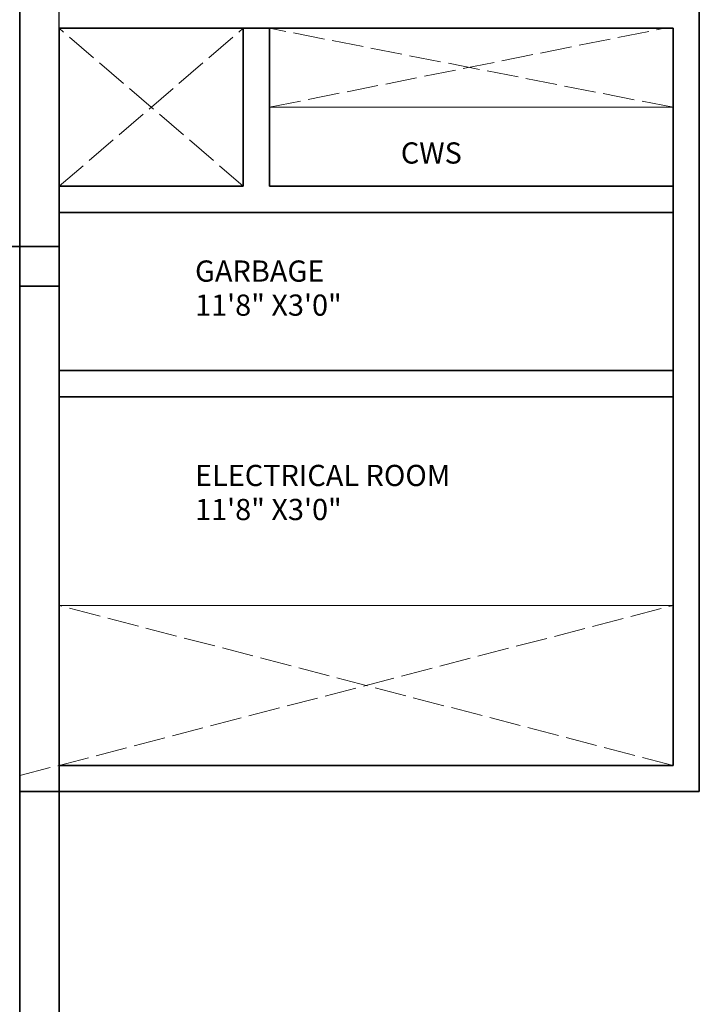
# Model space of a CAD drawing. Units: inches. Extents: x -61 to 1599, y -1316 to 257.
# Tile 76 of 204: x 536 to 691, y -790 to -565. Entities that reach past the tile are written whole.
import ezdxf

# ---------------------------------------------------------------- set-up
doc = ezdxf.new("R2010")
doc.units = ezdxf.units.IN
doc.header["$MEASUREMENT"] = 0
doc.linetypes.add('ACAD_ISO02W100', pattern=[15, 12, -3])
for name, color, linetype, lineweight in [('A-ANNO-DIMS', 2, 'Continuous', 18), ('A-ANNO-SYMB', 1, 'Continuous', 18), ('A-AREA-IDEN', 1, 'Continuous', 18), ('A-FLOR-OPEN', 8, 'Continuous', 18), ('A-FLOR-OPEN-HIDN', 8, 'ACAD_ISO02W100', 13), ('WALLS', 4, 'Continuous', 35)]:
    doc.layers.add(name, color=color, linetype=linetype, lineweight=lineweight)
doc.styles.get("Standard").update_dxf_attribs({"font": 'arial.ttf'})
doc.dimstyles.get("Standard").update_dxf_attribs({"dimtxt": 0.18, "dimasz": 0.18, "dimexe": 0.18, "dimexo": 0.0625, "dimgap": 0.09, "dimtad": 0, "dimtih": 1, "dimtoh": 1, "dimdec": 0, "dimzin": 0, "dimdsep": 46, "dimlunit": 3, "dimtxsty": 'Standard', "dimcen": 0.09, "dimadec": 0, "dimazin": 0, "dimtfac": 1, "dimtdec": 0, "dimtofl": 0, "dimtmove": 0, "dimatfit": 3, "dimfxl": 1, "dimtolj": 1, "dimtzin": 0, "dimarcsym": 0})

# ---------------------------------------------------------------- blocks, each defined once
blk = doc.blocks.new('*D704')
at = {"layer": 'A-ANNO-DIMS', "color": 0, "lineweight": -2, "transparency": 16777216}
for p, q in [((491.83, -616.88), (491.83, 257.46)), ((492.01, 257.28), (517.87, 257.28)), ((544.52, 257.28), (518.66, 257.28)), ((544.7, -616.88), (544.7, 257.46))]:
    blk.add_line(p, q, dxfattribs=at)
at = {"layer": 'A-ANNO-DIMS', "color": 0, "transparency": 16777216}
for points in [[(492.01, 257.31), (492.01, 257.25), (491.83, 257.28)], [(544.52, 257.31), (544.52, 257.25), (544.7, 257.28)]]:
    blk.add_solid(points, dxfattribs=at)
at = {"layer": 'DEFPOINTS', "color": 0, "transparency": 16777216}
for p in [(544.7, 257.28), (491.83, -616.94), (544.7, -616.94)]:
    blk.add_point(p, dxfattribs=at)
at = {"layer": 'A-ANNO-DIMS', "color": 0, "transparency": 16777216, "insert": (518.27, 257.28), "char_height": 0.18, "attachment_point": 5}
blk.add_mtext('\\A1;52.87', dxfattribs=at)

msp = doc.modelspace()

# ---------------------------------------------------------------- linework, layer by layer
at = {"layer": 'A-FLOR-OPEN'}
for p, q in [((592.7028, -585.169), (684.7028, -585.169)), ((544.7028, -698.7314), (684.7028, -698.7314))]:
    msp.add_line(p, q, dxfattribs=at)
at = {"layer": 'A-FLOR-OPEN-HIDN', "ltscale": 0.6}
for p, q in [((544.7028, -603.169), (586.7028, -567.169)), ((586.7028, -603.169), (544.7028, -567.169)), ((592.7028, -585.169), (682.7028, -567.169)), ((684.7028, -585.169), (592.7028, -567.169)), ((535.7028, -737.5114), (684.7028, -698.7314)), ((684.7028, -735.169), (544.7028, -698.7314))]:
    msp.add_line(p, q, dxfattribs=at)
at = {"layer": 'WALLS'}
for p, q in [((535.7028, -561.169), (535.7028, -741.169)), ((690.7028, -741.169), (690.7028, -561.169)), ((544.7028, -567.169), (684.7028, -567.169)), ((544.7028, -603.169), (544.7028, -567.169)), ((586.7028, -603.169), (586.7028, -567.169)), ((592.7028, -603.169), (592.7028, -567.169)), ((684.7028, -567.169), (679.7028, -567.169)), ((684.7028, -567.169), (679.7028, -567.169)), ((684.7028, -645.169), (684.7028, -567.169)), ((544.7028, -603.169), (586.7028, -603.169)), ((544.7028, -603.169), (544.7028, -609.169)), ((592.7028, -603.169), (684.7028, -603.169)), ((544.7028, -609.169), (684.7028, -609.169)), ((544.7028, -645.169), (544.7028, -609.169)), ((544.7028, -616.9446), (14.7028, -616.9446)), ((535.7028, -625.9446), (544.7028, -625.9446)), ((544.7028, -645.169), (684.7028, -645.169)), ((544.7028, -645.169), (544.7028, -741.169)), ((684.7028, -645.169), (684.7028, -735.169)), ((544.7028, -651.169), (684.7028, -651.169)), ((544.7028, -735.169), (684.7028, -735.169)), ((535.7028, -741.169), (690.7028, -741.169)), ((535.7028, -1215.9446), (535.7028, -741.169)), ((544.7028, -1215.9446), (544.7028, -741.169))]:
    msp.add_line(p, q, dxfattribs=at)

# ---------------------------------------------------------------- texts
at = {"layer": 'A-ANNO-SYMB'}
msp.add_text('CWS', height=4.8321, dxfattribs=at).set_placement((622.6217, -598.008))
at = {"layer": 'A-AREA-IDEN'}
for s, height, p in [('GARBAGE', 4.8321, (575.6945, -624.9257)), ('11\'8" X3\'0"', 4.832098, (575.6945, -632.688)), ('ELECTRICAL ROOM', 4.832098, (575.6945, -671.5087)), ('11\'8" X3\'0"', 4.832098, (575.6945, -679.271))]:
    msp.add_text(s, height=height, dxfattribs=at).set_placement(p)

# ---------------------------------------------------------------- dimensions: what is measured, and where the dimension line sits
at = {"layer": 'A-ANNO-DIMS'}
dim = msp.add_linear_dim(base=(544.7028, 257.2771), p1=(491.8327, -616.9446), p2=(544.7028, -616.9446), dimstyle='Standard', override={"dimdec": 2, "dimlfac": 1, "dimrnd": 0, "dimzin": 0, "dimdsep": 46, "dimlunit": 2}, dxfattribs=at)
dim.commit()
dim.dimension.update_dxf_attribs({"geometry": '*D704', "text_midpoint": (518.2677, 257.2771)})

doc.saveas('drawing.dxf')
